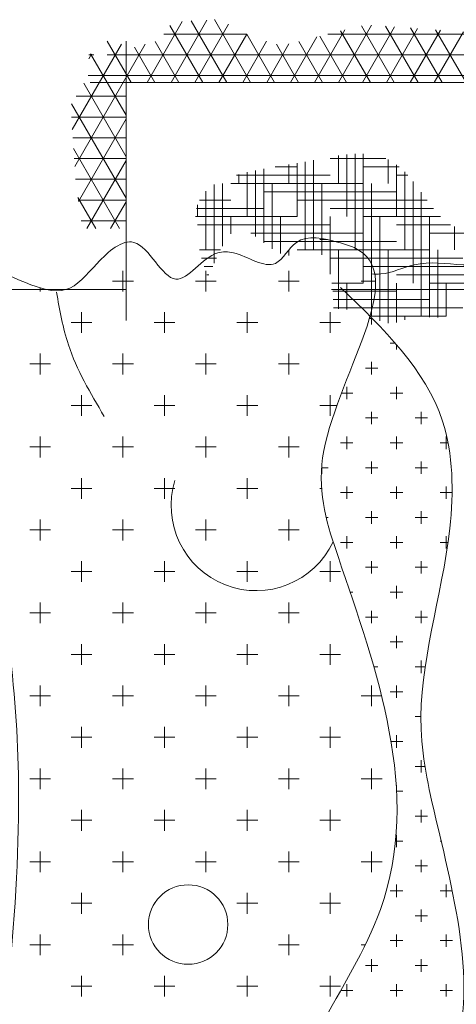
# Model space of a CAD drawing. Units: inches. Extents: x 3731 to 4318, y 1310 to 2388.
# Tile 37 of 57: x 3870 to 3897, y 2243 to 2304. Entities that reach past the tile are written whole.
import ezdxf

# ---------------------------------------------------------------- set-up
doc = ezdxf.new("R2010")
doc.units = ezdxf.units.IN
doc.layers.add('A-FURN', color=8, linetype='Continuous', lineweight=13)

# ---------------------------------------------------------------- blocks, each defined once
blk = doc.blocks.new('A$C200C7901')
for p, q in [((2, 1.6055), (2, 2.3334)), ((1.1379, 1.7195), (1.1379, 1.7508)), ((1.1222, 1.7352), (1.1535, 1.7352)), ((1.9972, 1.7352), (2.0027, 1.7352)), ((1.9972, 1.7352), (2.0027, 1.7352)), ((2, 1.6963), (2, 1.7248)), ((2, 1.6963), (2, 1.7248)), ((2.3121, 1.6596), (2.3121, 0.0201)), ((1.0129, 1.5945), (1.0129, 1.6258)), ((1.0129, 1.5945), (1.0129, 1.6258)), ((1.9533, 1.6055), (2.3741, 1.6055)), ((1.9533, 1.6055), (2.3741, 1.6055)), ((1.0754, 1.5625), (1.0754, 1.5633)), ((1.0754, 1.5625), (1.0754, 1.5633)), ((2, 0.2957), (2, 1.2957)), ((2.0224, 0.9977), (2.0224, 1.1977)), ((2.0224, 0.9977), (2.0224, 1.1977))]:
    blk.add_line(p, q)
at = {"linetype": 'ByBlock'}
for p, q in [((1.0129, 1.7195), (1.0129, 1.7508)), ((1.0129, 1.7195), (1.0129, 1.7508)), ((1.1379, 1.7195), (1.1379, 1.7508)), ((1.2629, 1.7195), (1.2629, 1.7508)), ((1.2629, 1.7195), (1.2629, 1.7508)), ((1.3879, 1.7195), (1.3879, 1.7508)), ((1.3879, 1.7195), (1.3879, 1.7508)), ((1.5129, 1.7195), (1.5129, 1.7508)), ((1.5129, 1.7195), (1.5129, 1.7508)), ((1.6379, 1.7195), (1.6379, 1.7508)), ((1.6379, 1.7195), (1.6379, 1.7508)), ((1.7629, 1.7195), (1.7629, 1.7508)), ((1.7629, 1.7195), (1.7629, 1.7508)), ((1.8879, 1.7195), (1.8879, 1.7508)), ((1.8879, 1.7195), (1.8879, 1.7508)), ((0.9972, 1.7352), (1.0285, 1.7352)), ((0.9972, 1.7352), (1.0285, 1.7352)), ((1.1222, 1.7352), (1.1535, 1.7352)), ((1.2472, 1.7352), (1.2785, 1.7352)), ((1.2472, 1.7352), (1.2785, 1.7352)), ((1.3722, 1.7352), (1.4035, 1.7352)), ((1.3722, 1.7352), (1.4035, 1.7352)), ((1.4972, 1.7352), (1.5285, 1.7352)), ((1.4972, 1.7352), (1.5285, 1.7352)), ((1.6222, 1.7352), (1.6535, 1.7352)), ((1.6222, 1.7352), (1.6535, 1.7352)), ((1.7472, 1.7352), (1.7785, 1.7352)), ((1.7472, 1.7352), (1.7785, 1.7352)), ((1.8722, 1.7352), (1.9035, 1.7352)), ((1.8722, 1.7352), (1.9035, 1.7352)), ((0.9504, 1.657), (0.9504, 1.6883)), ((0.9504, 1.657), (0.9504, 1.6883)), ((1.0754, 1.657), (1.0754, 1.6883)), ((1.0754, 1.657), (1.0754, 1.6883)), ((1.2004, 1.657), (1.2004, 1.6883)), ((1.2004, 1.657), (1.2004, 1.6883)), ((1.3254, 1.657), (1.3254, 1.6883)), ((1.3254, 1.657), (1.3254, 1.6883)), ((1.4504, 1.657), (1.4504, 1.6883)), ((1.4504, 1.657), (1.4504, 1.6883)), ((1.5754, 1.657), (1.5754, 1.6883)), ((1.5754, 1.657), (1.5754, 1.6883)), ((1.7004, 1.657), (1.7004, 1.6883)), ((1.7004, 1.657), (1.7004, 1.6883)), ((1.8254, 1.657), (1.8254, 1.6883)), ((1.8254, 1.657), (1.8254, 1.6883)), ((1.9504, 1.657), (1.9504, 1.6883)), ((1.9504, 1.657), (1.9504, 1.6883)), ((2.0919, 1.6152), (2.2125, 1.6848)), ((2.0919, 1.6152), (2.2125, 1.6848)), ((2.0919, 1.6513), (2.1386, 1.6782)), ((2.0919, 1.6513), (2.1386, 1.6782)), ((2.1327, 1.6773), (2.2571, 1.6055)), ((2.1327, 1.6773), (2.2571, 1.6055)), ((2.1349, 1.6055), (2.1349, 1.6777)), ((2.1349, 1.6055), (2.1349, 1.6777)), ((2.1377, 1.6055), (2.2798, 1.6876)), ((2.1377, 1.6055), (2.2798, 1.6876)), ((2.1662, 1.6055), (2.1662, 1.6817)), ((2.1662, 1.6055), (2.1662, 1.6817)), ((2.1854, 1.683), (2.3697, 1.5766)), ((2.1854, 1.683), (2.3697, 1.5766)), ((2.1974, 1.6055), (2.1974, 1.6838)), ((2.1974, 1.6055), (2.1974, 1.6838)), ((2.2287, 1.6055), (2.2287, 1.6859)), ((2.2287, 1.6055), (2.2287, 1.6859)), ((2.2414, 1.6868), (2.3699, 1.6126)), ((2.2414, 1.6868), (2.3699, 1.6126)), ((2.2599, 1.6055), (2.2599, 1.688)), ((2.2599, 1.6055), (2.2599, 1.688)), ((2.2912, 1.6055), (2.2912, 1.6809)), ((2.2912, 1.6055), (2.2912, 1.6809)), ((0.9347, 1.6727), (0.966, 1.6727)), ((0.9347, 1.6727), (0.966, 1.6727)), ((1.0597, 1.6727), (1.091, 1.6727)), ((1.0597, 1.6727), (1.091, 1.6727)), ((1.1847, 1.6727), (1.216, 1.6727)), ((1.1847, 1.6727), (1.216, 1.6727)), ((1.3097, 1.6727), (1.341, 1.6727)), ((1.3097, 1.6727), (1.341, 1.6727)), ((1.4347, 1.6727), (1.466, 1.6727)), ((1.4347, 1.6727), (1.466, 1.6727)), ((1.5597, 1.6727), (1.591, 1.6727)), ((1.5597, 1.6727), (1.591, 1.6727)), ((1.6847, 1.6727), (1.716, 1.6727)), ((1.6847, 1.6727), (1.716, 1.6727)), ((1.8097, 1.6727), (1.841, 1.6727)), ((1.8097, 1.6727), (1.841, 1.6727)), ((1.9347, 1.6727), (1.966, 1.6727)), ((1.9347, 1.6727), (1.966, 1.6727)), ((2.0919, 1.6649), (2.1946, 1.6055)), ((2.0919, 1.6649), (2.1946, 1.6055)), ((2.1037, 1.6055), (2.1037, 1.673)), ((2.1037, 1.6055), (2.1037, 1.673)), ((2.2002, 1.6055), (2.3109, 1.6694)), ((2.2002, 1.6055), (2.3109, 1.6694)), ((2.3224, 0.0468), (2.3224, 1.6627)), ((2.3224, 0.0468), (2.3224, 1.6627)), ((2.3476, 1.6616), (2.3547, 1.6575)), ((2.3476, 1.6616), (2.3547, 1.6575)), ((2.3537, 1.6539), (2.3537, 1.6616)), ((2.3537, 1.6539), (2.3537, 1.6616)), ((2.2627, 1.6055), (2.3551, 1.6589)), ((2.2627, 1.6055), (2.3551, 1.6589)), ((2.3121, 1.598), (2.3745, 1.634)), ((2.3121, 1.598), (2.3745, 1.634)), ((2.3537, 0.0056), (2.3537, 1.634)), ((2.3537, 0.0056), (2.3537, 1.634)), ((1.1379, 1.5945), (1.1379, 1.6258)), ((1.1379, 1.5945), (1.1379, 1.6258)), ((1.2629, 1.5945), (1.2629, 1.6258)), ((1.2629, 1.5945), (1.2629, 1.6258)), ((1.3879, 1.5945), (1.3879, 1.6258)), ((1.3879, 1.5945), (1.3879, 1.6258)), ((1.5129, 1.5945), (1.5129, 1.6258)), ((1.5129, 1.5945), (1.5129, 1.6258)), ((1.6379, 1.5945), (1.6379, 1.6258)), ((1.6379, 1.5945), (1.6379, 1.6258)), ((1.7629, 1.5945), (1.7629, 1.6258)), ((1.7629, 1.5945), (1.7629, 1.6258)), ((1.8879, 1.5945), (1.8879, 1.6258)), ((1.8879, 1.5945), (1.8879, 1.6258)), ((2.0129, 1.5945), (2.0129, 1.6258)), ((2.0129, 1.5945), (2.0129, 1.6258)), ((2.0919, 1.6288), (2.1321, 1.6055)), ((2.0919, 1.6288), (2.1321, 1.6055)), ((0.9972, 1.6102), (1.0285, 1.6102)), ((0.9972, 1.6102), (1.0285, 1.6102)), ((1.1222, 1.6102), (1.1535, 1.6102)), ((1.1222, 1.6102), (1.1535, 1.6102)), ((1.2472, 1.6102), (1.2785, 1.6102)), ((1.2472, 1.6102), (1.2785, 1.6102)), ((1.3722, 1.6102), (1.4035, 1.6102)), ((1.3722, 1.6102), (1.4035, 1.6102)), ((1.4972, 1.6102), (1.5285, 1.6102)), ((1.4972, 1.6102), (1.5285, 1.6102)), ((1.6222, 1.6102), (1.6535, 1.6102)), ((1.6222, 1.6102), (1.6535, 1.6102)), ((1.7472, 1.6102), (1.7785, 1.6102)), ((1.7472, 1.6102), (1.7785, 1.6102)), ((1.8722, 1.6102), (1.9035, 1.6102)), ((1.8722, 1.6102), (1.9035, 1.6102)), ((1.9972, 1.6102), (2.0285, 1.6102)), ((1.9972, 1.6102), (2.0285, 1.6102)), ((2.3121, 1.5619), (2.3654, 1.5926)), ((2.3121, 1.5619), (2.3654, 1.5926)), ((2.3121, 1.5738), (2.404, 1.5208)), ((2.3121, 1.5738), (2.404, 1.5208)), ((0.9504, 1.532), (0.9504, 1.5633)), ((0.9504, 1.532), (0.9504, 1.5633)), ((1.2004, 1.532), (1.2004, 1.5633)), ((1.2004, 1.532), (1.2004, 1.5633)), ((1.3254, 1.532), (1.3254, 1.5633)), ((1.3254, 1.532), (1.3254, 1.5633)), ((1.4504, 1.532), (1.4504, 1.5633)), ((1.4504, 1.532), (1.4504, 1.5633)), ((1.5754, 1.532), (1.5754, 1.5633)), ((1.5754, 1.532), (1.5754, 1.5633)), ((1.7004, 1.532), (1.7004, 1.5633)), ((1.7004, 1.532), (1.7004, 1.5633)), ((1.8254, 1.532), (1.8254, 1.5633)), ((1.8254, 1.532), (1.8254, 1.5633)), ((1.9504, 1.532), (1.9504, 1.5633)), ((1.9504, 1.532), (1.9504, 1.5633)), ((2.3121, 1.5258), (2.3739, 1.5615)), ((2.3121, 1.5258), (2.3739, 1.5615)), ((0.9347, 1.5477), (0.966, 1.5477)), ((0.9347, 1.5477), (0.966, 1.5477)), ((1.1847, 1.5477), (1.216, 1.5477)), ((1.1847, 1.5477), (1.216, 1.5477)), ((1.3097, 1.5477), (1.341, 1.5477)), ((1.3097, 1.5477), (1.341, 1.5477)), ((1.4347, 1.5477), (1.466, 1.5477)), ((1.4347, 1.5477), (1.466, 1.5477)), ((1.5597, 1.5477), (1.591, 1.5477)), ((1.5597, 1.5477), (1.591, 1.5477)), ((1.6847, 1.5477), (1.716, 1.5477)), ((1.6847, 1.5477), (1.716, 1.5477)), ((1.8097, 1.5477), (1.841, 1.5477)), ((1.8097, 1.5477), (1.841, 1.5477)), ((1.9347, 1.5477), (1.966, 1.5477)), ((1.9347, 1.5477), (1.966, 1.5477)), ((2.3849, 1.4236), (2.3849, 1.5486)), ((2.3849, 1.4236), (2.3849, 1.5486)), ((2.3121, 1.4897), (2.3979, 1.5393)), ((2.3121, 1.4897), (2.3979, 1.5393)), ((2.3121, 1.5377), (2.406, 1.4835)), ((2.3121, 1.5377), (2.406, 1.4835)), ((1.1379, 1.4695), (1.1379, 1.5008)), ((1.1379, 1.4695), (1.1379, 1.5008)), ((1.2629, 1.4695), (1.2629, 1.5008)), ((1.2629, 1.4695), (1.2629, 1.5008)), ((1.3879, 1.4695), (1.3879, 1.5008)), ((1.3879, 1.4695), (1.3879, 1.5008)), ((1.5129, 1.4695), (1.5129, 1.5008)), ((1.5129, 1.4695), (1.5129, 1.5008)), ((1.6379, 1.4695), (1.6379, 1.5008)), ((1.6379, 1.4695), (1.6379, 1.5008)), ((1.7629, 1.4695), (1.7629, 1.5008)), ((1.7629, 1.4695), (1.7629, 1.5008)), ((1.8879, 1.4695), (1.8879, 1.5008)), ((1.8879, 1.4695), (1.8879, 1.5008)), ((2.0129, 1.4695), (2.0129, 1.5008)), ((2.0129, 1.4695), (2.0129, 1.5008)), ((2.1099, 1.3477), (2.1099, 1.5009)), ((2.1099, 1.3477), (2.1099, 1.5009)), ((2.1224, 1.3977), (2.1224, 1.4992)), ((2.1224, 1.3977), (2.1224, 1.4992)), ((2.3121, 1.4537), (2.4047, 1.5071)), ((2.3121, 1.4537), (2.4047, 1.5071)), ((2.3121, 1.5016), (2.3997, 1.4511)), ((2.3121, 1.5016), (2.3997, 1.4511)), ((1.1222, 1.4852), (1.1535, 1.4852)), ((1.1222, 1.4852), (1.1535, 1.4852)), ((1.2472, 1.4852), (1.2785, 1.4852)), ((1.2472, 1.4852), (1.2785, 1.4852)), ((1.3722, 1.4852), (1.4035, 1.4852)), ((1.3722, 1.4852), (1.4035, 1.4852)), ((1.4972, 1.4852), (1.5285, 1.4852)), ((1.4972, 1.4852), (1.5285, 1.4852)), ((1.6222, 1.4852), (1.6535, 1.4852)), ((1.6222, 1.4852), (1.6535, 1.4852)), ((1.7472, 1.4852), (1.7785, 1.4852)), ((1.7472, 1.4852), (1.7785, 1.4852)), ((1.8722, 1.4852), (1.9035, 1.4852)), ((1.8722, 1.4852), (1.9035, 1.4852)), ((1.9972, 1.4852), (2.0285, 1.4852)), ((1.9972, 1.4852), (2.0285, 1.4852)), ((2.0224, 1.4805), (2.0224, 1.4839)), ((2.0224, 1.4805), (2.0224, 1.4839)), ((2.0349, 1.4748), (2.0349, 1.4879)), ((2.0349, 1.4748), (2.0349, 1.4879)), ((2.0474, 1.4691), (2.0474, 1.4915)), ((2.0474, 1.4691), (2.0474, 1.4915)), ((2.0599, 1.4631), (2.0599, 1.4948)), ((2.0599, 1.4631), (2.0599, 1.4948)), ((2.0599, 1.4852), (2.1484, 1.4852)), ((2.0599, 1.4852), (2.1484, 1.4852)), ((2.0974, 1.2977), (2.0974, 1.4977)), ((2.0974, 1.2977), (2.0974, 1.4977)), ((2.1099, 1.4977), (2.1279, 1.4977)), ((2.1099, 1.4977), (2.1279, 1.4977)), ((2.1349, 1.4477), (2.1349, 1.4949)), ((2.1349, 1.4477), (2.1349, 1.4949)), ((2.0397, 1.4727), (2.1581, 1.4727)), ((2.0397, 1.4727), (2.1581, 1.4727)), ((2.3121, 1.4176), (2.4067, 1.4721)), ((2.3121, 1.4176), (2.4067, 1.4721)), ((2.0656, 1.4602), (2.1599, 1.4602)), ((2.0656, 1.4602), (2.1599, 1.4602)), ((2.3121, 1.4655), (2.3849, 1.4235)), ((2.3121, 1.4655), (2.3849, 1.4235)), ((2.084, 1.4477), (2.1099, 1.4477)), ((2.084, 1.4477), (2.1099, 1.4477)), ((2.0849, 1.4468), (2.0849, 1.4477)), ((2.0849, 1.4468), (2.0849, 1.4477)), ((2.1599, 1.2477), (2.1599, 1.4477)), ((2.1599, 1.2477), (2.1599, 1.4477)), ((2.1724, 1.2977), (2.1724, 1.439)), ((2.1724, 1.2977), (2.1724, 1.439)), ((0.9504, 1.407), (0.9504, 1.4383)), ((0.9504, 1.407), (0.9504, 1.4383)), ((1.0754, 1.407), (1.0754, 1.4383)), ((1.0754, 1.407), (1.0754, 1.4383)), ((1.2004, 1.407), (1.2004, 1.4383)), ((1.2004, 1.407), (1.2004, 1.4383)), ((1.3254, 1.407), (1.3254, 1.4383)), ((1.3254, 1.407), (1.3254, 1.4383)), ((1.4504, 1.407), (1.4504, 1.4383)), ((1.4504, 1.407), (1.4504, 1.4383)), ((1.5754, 1.407), (1.5754, 1.4383)), ((1.5754, 1.407), (1.5754, 1.4383)), ((1.7004, 1.407), (1.7004, 1.4383)), ((1.7004, 1.407), (1.7004, 1.4383)), ((1.8254, 1.407), (1.8254, 1.4383)), ((1.8254, 1.407), (1.8254, 1.4383)), ((1.9504, 1.407), (1.9504, 1.4383)), ((1.9504, 1.407), (1.9504, 1.4383)), ((2.1599, 1.4352), (2.1735, 1.4352)), ((2.1599, 1.4352), (2.1735, 1.4352)), ((2.3121, 1.4294), (2.3741, 1.3937)), ((2.3121, 1.4294), (2.3741, 1.3937)), ((0.9347, 1.4227), (0.966, 1.4227)), ((0.9347, 1.4227), (0.966, 1.4227)), ((1.0597, 1.4227), (1.091, 1.4227)), ((1.0597, 1.4227), (1.091, 1.4227)), ((1.1847, 1.4227), (1.216, 1.4227)), ((1.1847, 1.4227), (1.216, 1.4227)), ((1.3097, 1.4227), (1.341, 1.4227)), ((1.3097, 1.4227), (1.341, 1.4227)), ((1.4347, 1.4227), (1.466, 1.4227)), ((1.4347, 1.4227), (1.466, 1.4227)), ((1.5597, 1.4227), (1.591, 1.4227)), ((1.5597, 1.4227), (1.591, 1.4227)), ((1.6847, 1.4227), (1.716, 1.4227)), ((1.6847, 1.4227), (1.716, 1.4227)), ((1.8097, 1.4227), (1.841, 1.4227)), ((1.8097, 1.4227), (1.841, 1.4227)), ((1.9347, 1.4227), (1.966, 1.4227)), ((1.9347, 1.4227), (1.966, 1.4227)), ((2.08, 1.4102), (2.1795, 1.4102)), ((2.08, 1.4102), (2.1795, 1.4102)), ((2.0849, 1.2477), (2.0849, 1.4171)), ((2.0849, 1.2477), (2.0849, 1.4171)), ((2.1099, 1.4227), (2.1767, 1.4227)), ((2.1099, 1.4227), (2.1767, 1.4227)), ((2.3121, 1.3815), (2.3848, 1.4235)), ((2.3121, 1.3815), (2.3848, 1.4235)), ((2.0703, 1.3977), (2.1819, 1.3977)), ((2.0703, 1.3977), (2.1819, 1.3977)), ((2.0724, 1.1977), (2.0724, 1.3977)), ((2.0724, 1.1977), (2.0724, 1.3977)), ((2.1474, 1.1977), (2.1474, 1.3977)), ((2.1474, 1.1977), (2.1474, 1.3977)), ((2.0612, 1.3852), (2.1599, 1.3852)), ((2.0612, 1.3852), (2.1599, 1.3852)), ((2.1849, 1.3477), (2.1849, 1.3808)), ((2.1849, 1.3477), (2.1849, 1.3808)), ((2.3121, 1.3934), (2.3703, 1.3598)), ((2.3121, 1.3934), (2.3703, 1.3598)), ((1.0129, 1.3445), (1.0129, 1.3758)), ((1.0129, 1.3445), (1.0129, 1.3758)), ((1.1379, 1.3445), (1.1379, 1.3758)), ((1.1379, 1.3445), (1.1379, 1.3758)), ((1.2629, 1.3445), (1.2629, 1.3758)), ((1.2629, 1.3445), (1.2629, 1.3758)), ((1.3879, 1.3445), (1.3879, 1.3758)), ((1.3879, 1.3445), (1.3879, 1.3758)), ((1.5129, 1.3445), (1.5129, 1.3758)), ((1.5129, 1.3445), (1.5129, 1.3758)), ((1.6379, 1.3445), (1.6379, 1.3758)), ((1.6379, 1.3445), (1.6379, 1.3758)), ((1.7629, 1.3445), (1.7629, 1.3758)), ((1.7629, 1.3445), (1.7629, 1.3758)), ((1.8879, 1.3445), (1.8879, 1.3758)), ((1.8879, 1.3445), (1.8879, 1.3758)), ((2.0129, 1.3445), (2.0129, 1.3758)), ((2.0129, 1.3445), (2.0129, 1.3758)), ((2.0545, 1.3727), (2.1099, 1.3727)), ((2.0545, 1.3727), (2.1099, 1.3727)), ((2.3121, 1.3454), (2.37, 1.3788)), ((2.3121, 1.3454), (2.37, 1.3788)), ((0.9972, 1.3602), (1.0285, 1.3602)), ((0.9972, 1.3602), (1.0285, 1.3602)), ((1.1222, 1.3602), (1.1535, 1.3602)), ((1.1222, 1.3602), (1.1535, 1.3602)), ((1.2472, 1.3602), (1.2785, 1.3602)), ((1.2472, 1.3602), (1.2785, 1.3602)), ((1.3722, 1.3602), (1.4035, 1.3602)), ((1.3722, 1.3602), (1.4035, 1.3602)), ((1.4972, 1.3602), (1.5285, 1.3602)), ((1.4972, 1.3602), (1.5285, 1.3602)), ((1.6222, 1.3602), (1.6535, 1.3602)), ((1.6222, 1.3602), (1.6535, 1.3602)), ((1.7472, 1.3602), (1.7785, 1.3602)), ((1.7472, 1.3602), (1.7785, 1.3602)), ((1.8722, 1.3602), (1.9035, 1.3602)), ((1.8722, 1.3602), (1.9035, 1.3602)), ((1.9972, 1.3602), (2.0285, 1.3602)), ((1.9972, 1.3602), (2.0285, 1.3602)), ((2.0515, 1.3602), (2.0599, 1.3602)), ((2.0515, 1.3602), (2.0599, 1.3602)), ((2.1599, 1.3602), (2.1883, 1.3602)), ((2.1599, 1.3602), (2.1883, 1.3602)), ((2.3121, 1.3573), (2.3808, 1.3176)), ((2.3121, 1.3573), (2.3808, 1.3176)), ((2.0599, 1.1477), (2.0599, 1.3477)), ((2.0599, 1.1477), (2.0599, 1.3477)), ((2.0599, 1.3352), (2.1926, 1.3352)), ((2.0599, 1.3352), (2.1926, 1.3352)), ((2.1099, 1.3477), (2.1904, 1.3477)), ((2.1099, 1.3477), (2.1904, 1.3477)), ((2.1349, 1.1515), (2.1349, 1.3477)), ((2.1349, 1.1515), (2.1349, 1.3477)), ((2.3121, 1.3093), (2.374, 1.345)), ((2.3121, 1.3093), (2.374, 1.345)), ((2.0594, 1.3227), (2.195, 1.3227)), ((2.0594, 1.3227), (2.195, 1.3227)), ((2.3121, 1.3212), (2.3914, 1.2754)), ((2.3121, 1.3212), (2.3914, 1.2754)), ((0.9504, 1.282), (0.9504, 1.3133)), ((0.9504, 1.282), (0.9504, 1.3133)), ((1.0754, 1.282), (1.0754, 1.3133)), ((1.0754, 1.282), (1.0754, 1.3133)), ((1.2004, 1.282), (1.2004, 1.3133)), ((1.2004, 1.282), (1.2004, 1.3133)), ((1.3254, 1.282), (1.3254, 1.3133)), ((1.3254, 1.282), (1.3254, 1.3133)), ((1.4504, 1.282), (1.4504, 1.3133)), ((1.4504, 1.282), (1.4504, 1.3133)), ((1.5754, 1.282), (1.5754, 1.3133)), ((1.5754, 1.282), (1.5754, 1.3133)), ((1.7004, 1.3106), (1.7004, 1.3133)), ((1.7004, 1.3106), (1.7004, 1.3133)), ((1.7222, 1.3102), (1.7369, 1.3102)), ((1.7222, 1.3102), (1.7369, 1.3102)), ((1.7316, 1.3008), (1.7316, 1.3106)), ((1.7316, 1.3008), (1.7316, 1.3106)), ((1.8254, 1.2876), (1.8254, 1.3133)), ((1.8254, 1.2876), (1.8254, 1.3133)), ((1.9504, 1.282), (1.9504, 1.3133)), ((1.9504, 1.282), (1.9504, 1.3133)), ((2.0524, 1.3102), (2.1599, 1.3102)), ((2.0524, 1.3102), (2.1599, 1.3102)), ((2.0754, 1.3017), (2.0754, 1.3133)), ((2.0754, 1.3017), (2.0754, 1.3133)), ((2.3121, 1.2732), (2.3819, 1.3135)), ((2.3121, 1.2732), (2.3819, 1.3135)), ((0.9347, 1.2977), (0.966, 1.2977)), ((0.9347, 1.2977), (0.966, 1.2977)), ((1.0597, 1.2977), (1.091, 1.2977)), ((1.0597, 1.2977), (1.091, 1.2977)), ((1.1847, 1.2977), (1.216, 1.2977)), ((1.1847, 1.2977), (1.216, 1.2977)), ((1.3097, 1.2977), (1.341, 1.2977)), ((1.3097, 1.2977), (1.341, 1.2977)), ((1.4347, 1.2977), (1.466, 1.2977)), ((1.4347, 1.2977), (1.466, 1.2977)), ((1.5597, 1.2977), (1.591, 1.2977)), ((1.5597, 1.2977), (1.591, 1.2977)), ((1.6566, 1.3008), (1.6566, 1.3036)), ((1.6566, 1.3008), (1.6566, 1.3036)), ((1.8097, 1.2977), (1.841, 1.2977)), ((1.8097, 1.2977), (1.841, 1.2977)), ((1.9347, 1.2977), (1.966, 1.2977)), ((1.9347, 1.2977), (1.966, 1.2977)), ((1.9724, 1.0977), (1.9724, 1.2927)), ((1.9724, 1.0977), (1.9724, 1.2927)), ((1.9849, 1.1477), (1.9849, 1.293)), ((1.9849, 1.1477), (1.9849, 1.293)), ((1.9974, 1.1977), (1.9974, 1.2939)), ((1.9974, 1.1977), (1.9974, 1.2939)), ((2.0099, 1.2477), (2.0099, 1.2953)), ((2.0099, 1.2477), (2.0099, 1.2953)), ((2.023, 1.2977), (2.1099, 1.2977)), ((2.023, 1.2977), (2.1099, 1.2977)), ((2.0474, 1.0977), (2.0474, 1.2977)), ((2.0474, 1.0977), (2.0474, 1.2977)), ((2.0597, 1.2977), (2.0744, 1.2977)), ((2.0597, 1.2977), (2.0744, 1.2977)), ((2.1224, 1.1421), (2.1224, 1.2977)), ((2.1224, 1.1421), (2.1224, 1.2977)), ((2.1974, 1.2135), (2.1974, 1.2977)), ((2.1974, 1.2135), (2.1974, 1.2977)), ((2.3849, 1.0607), (2.3849, 1.3013)), ((2.3849, 1.0607), (2.3849, 1.3013)), ((0.9441, 1.2633), (0.9441, 1.2816)), ((0.9441, 1.2633), (0.9441, 1.2816)), ((1.6191, 1.2633), (1.6191, 1.282)), ((1.6191, 1.2633), (1.6191, 1.282)), ((1.6941, 1.2633), (1.6941, 1.282)), ((1.6941, 1.2633), (1.6941, 1.282)), ((1.7691, 1.2633), (1.7691, 1.282)), ((1.7691, 1.2633), (1.7691, 1.282)), ((1.8441, 1.2633), (1.8441, 1.2806)), ((1.8441, 1.2633), (1.8441, 1.2806)), ((1.9711, 1.2852), (2.0599, 1.2852)), ((1.9711, 1.2852), (2.0599, 1.2852)), ((2.1599, 1.2852), (2.2018, 1.2852)), ((2.1599, 1.2852), (2.2018, 1.2852)), ((2.3121, 1.2851), (2.3985, 1.2352)), ((2.3121, 1.2851), (2.3985, 1.2352)), ((2.3121, 1.2371), (2.3898, 1.282)), ((2.3121, 1.2371), (2.3898, 1.282)), ((0.9347, 1.2727), (0.9535, 1.2727)), ((0.9347, 1.2727), (0.9535, 1.2727)), ((1.5441, 1.2633), (1.5441, 1.2675)), ((1.5441, 1.2633), (1.5441, 1.2675)), ((1.6097, 1.2727), (1.6285, 1.2727)), ((1.6097, 1.2727), (1.6285, 1.2727)), ((1.6847, 1.2727), (1.7035, 1.2727)), ((1.6847, 1.2727), (1.7035, 1.2727)), ((1.7597, 1.2727), (1.7785, 1.2727)), ((1.7597, 1.2727), (1.7785, 1.2727)), ((1.8347, 1.2727), (1.8535, 1.2727)), ((1.8347, 1.2727), (1.8535, 1.2727)), ((1.97, 1.2727), (2.0099, 1.2727)), ((1.97, 1.2727), (2.0099, 1.2727)), ((2.1099, 1.2727), (2.2034, 1.2727)), ((2.1099, 1.2727), (2.2034, 1.2727)), ((1.0129, 1.2448), (1.0129, 1.2508)), ((1.0129, 1.2448), (1.0129, 1.2508)), ((1.1379, 1.2195), (1.1379, 1.2508)), ((1.1379, 1.2195), (1.1379, 1.2508)), ((1.2629, 1.2195), (1.2629, 1.2508)), ((1.2629, 1.2195), (1.2629, 1.2508)), ((1.3879, 1.2202), (1.3879, 1.2508)), ((1.3879, 1.2202), (1.3879, 1.2508)), ((2.0099, 1.2477), (2.2045, 1.2477)), ((2.0099, 1.2477), (2.2045, 1.2477)), ((2.0129, 1.2293), (2.0129, 1.2508)), ((2.0129, 1.2293), (2.0129, 1.2508)), ((2.0349, 1.0477), (2.0349, 1.2477)), ((2.0349, 1.0477), (2.0349, 1.2477)), ((2.0599, 1.2602), (2.2044, 1.2602)), ((2.0599, 1.2602), (2.2044, 1.2602)), ((2.1099, 1.1315), (2.1099, 1.2477)), ((2.1099, 1.1315), (2.1099, 1.2477)), ((2.1849, 1.1935), (2.1849, 1.2477)), ((2.1849, 1.1935), (2.1849, 1.2477)), ((2.3121, 1.2011), (2.3976, 1.2504)), ((2.3121, 1.2011), (2.3976, 1.2504)), ((2.3121, 1.249), (2.396, 1.2006)), ((2.3121, 1.249), (2.396, 1.2006)), ((0.9722, 1.2352), (0.991, 1.2352)), ((0.9722, 1.2352), (0.991, 1.2352)), ((0.9816, 1.2258), (0.9816, 1.2445)), ((0.9816, 1.2258), (0.9816, 1.2445)), ((1.1222, 1.2352), (1.1535, 1.2352)), ((1.1222, 1.2352), (1.1535, 1.2352)), ((1.2472, 1.2352), (1.2785, 1.2352)), ((1.2472, 1.2352), (1.2785, 1.2352)), ((1.3722, 1.2352), (1.4035, 1.2352)), ((1.3722, 1.2352), (1.4035, 1.2352)), ((1.4316, 1.2258), (1.4316, 1.2318)), ((1.4316, 1.2258), (1.4316, 1.2318)), ((1.4972, 1.2352), (1.516, 1.2352)), ((1.4972, 1.2352), (1.516, 1.2352)), ((1.5066, 1.2258), (1.5066, 1.2445)), ((1.5066, 1.2258), (1.5066, 1.2445)), ((1.5722, 1.2352), (1.591, 1.2352)), ((1.5722, 1.2352), (1.591, 1.2352)), ((1.5816, 1.2258), (1.5816, 1.2445)), ((1.5816, 1.2258), (1.5816, 1.2445)), ((1.6472, 1.2352), (1.666, 1.2352)), ((1.6472, 1.2352), (1.666, 1.2352)), ((1.6566, 1.2258), (1.6566, 1.2445)), ((1.6566, 1.2258), (1.6566, 1.2445)), ((1.7222, 1.2352), (1.741, 1.2352)), ((1.7222, 1.2352), (1.741, 1.2352)), ((1.7316, 1.2258), (1.7316, 1.2445)), ((1.7316, 1.2258), (1.7316, 1.2445)), ((1.7972, 1.2352), (1.816, 1.2352)), ((1.7972, 1.2352), (1.816, 1.2352)), ((1.8066, 1.2258), (1.8066, 1.2445)), ((1.8066, 1.2258), (1.8066, 1.2445)), ((1.8722, 1.2352), (1.891, 1.2352)), ((1.8722, 1.2352), (1.891, 1.2352)), ((1.8816, 1.2258), (1.8816, 1.2445)), ((1.8816, 1.2258), (1.8816, 1.2445)), ((1.9472, 1.2352), (1.9574, 1.2352)), ((1.9472, 1.2352), (1.9574, 1.2352)), ((1.9566, 1.2344), (1.9566, 1.2385)), ((1.9566, 1.2344), (1.9566, 1.2385)), ((1.9599, 1.1228), (1.9599, 1.2373)), ((1.9599, 1.1228), (1.9599, 1.2373)), ((1.9599, 1.2352), (2.1599, 1.2352)), ((1.9599, 1.2352), (2.1599, 1.2352)), ((2, 1.2352), (2.0285, 1.2352)), ((2, 1.2352), (2.0285, 1.2352)), ((1.953, 1.2227), (2.1099, 1.2227)), ((1.953, 1.2227), (2.1099, 1.2227)), ((0.9441, 1.1883), (0.9441, 1.207)), ((0.9441, 1.1883), (0.9441, 1.207)), ((1.0191, 1.1883), (1.0191, 1.207)), ((1.0191, 1.1883), (1.0191, 1.207)), ((1.0941, 1.1883), (1.0941, 1.207)), ((1.0941, 1.1883), (1.0941, 1.207)), ((1.3191, 1.1883), (1.3191, 1.2059)), ((1.3191, 1.1883), (1.3191, 1.2059)), ((1.3941, 1.1883), (1.3941, 1.207)), ((1.3941, 1.1883), (1.3941, 1.207)), ((1.4691, 1.1883), (1.4691, 1.207)), ((1.4691, 1.1883), (1.4691, 1.207)), ((1.5441, 1.1883), (1.5441, 1.207)), ((1.5441, 1.1883), (1.5441, 1.207)), ((1.6191, 1.1883), (1.6191, 1.207)), ((1.6191, 1.1883), (1.6191, 1.207)), ((1.6941, 1.1883), (1.6941, 1.207)), ((1.6941, 1.1883), (1.6941, 1.207)), ((1.7691, 1.1883), (1.7691, 1.207)), ((1.7691, 1.1883), (1.7691, 1.207)), ((1.8441, 1.1883), (1.8441, 1.207)), ((1.8441, 1.1883), (1.8441, 1.207)), ((1.9191, 1.1995), (1.9191, 1.207)), ((1.9191, 1.1995), (1.9191, 1.207)), ((1.9495, 1.2102), (2.0599, 1.2102)), ((1.9495, 1.2102), (2.0599, 1.2102)), ((2.1599, 1.2102), (2.1959, 1.2102)), ((2.1599, 1.2102), (2.1959, 1.2102)), ((2.3121, 1.165), (2.397, 1.214)), ((2.3121, 1.165), (2.397, 1.214)), ((2.3121, 1.2129), (2.3935, 1.166)), ((2.3121, 1.2129), (2.3935, 1.166)), ((0.9347, 1.1977), (0.9535, 1.1977)), ((0.9347, 1.1977), (0.9535, 1.1977)), ((1.0097, 1.1977), (1.0285, 1.1977)), ((1.0097, 1.1977), (1.0285, 1.1977)), ((1.0847, 1.1977), (1.1035, 1.1977)), ((1.0847, 1.1977), (1.1035, 1.1977)), ((1.1597, 1.1977), (1.1785, 1.1977)), ((1.1597, 1.1977), (1.1785, 1.1977)), ((1.1691, 1.1883), (1.1691, 1.1991)), ((1.1691, 1.1883), (1.1691, 1.1991)), ((1.2441, 1.1883), (1.2441, 1.1976)), ((1.2441, 1.1883), (1.2441, 1.1976)), ((1.2452, 1.1977), (1.2535, 1.1977)), ((1.2452, 1.1977), (1.2535, 1.1977)), ((1.3097, 1.1977), (1.3285, 1.1977)), ((1.3097, 1.1977), (1.3285, 1.1977)), ((1.3847, 1.1977), (1.4035, 1.1977)), ((1.3847, 1.1977), (1.4035, 1.1977)), ((1.4597, 1.1977), (1.4785, 1.1977)), ((1.4597, 1.1977), (1.4785, 1.1977)), ((1.5347, 1.1977), (1.5535, 1.1977)), ((1.5347, 1.1977), (1.5535, 1.1977)), ((1.6097, 1.1977), (1.6285, 1.1977)), ((1.6097, 1.1977), (1.6285, 1.1977)), ((1.6847, 1.1977), (1.7035, 1.1977)), ((1.6847, 1.1977), (1.7035, 1.1977)), ((1.7597, 1.1977), (1.7785, 1.1977)), ((1.7597, 1.1977), (1.7785, 1.1977)), ((1.8347, 1.1977), (1.8535, 1.1977)), ((1.8347, 1.1977), (1.8535, 1.1977)), ((1.9097, 1.1977), (1.917, 1.1977)), ((1.9097, 1.1977), (1.917, 1.1977)), ((1.9506, 1.1977), (2.0099, 1.1977)), ((1.9506, 1.1977), (2.0099, 1.1977)), ((2.0974, 1.1161), (2.0974, 1.1977)), ((2.0974, 1.1161), (2.0974, 1.1977)), ((2.1099, 1.1977), (2.1882, 1.1977)), ((2.1099, 1.1977), (2.1882, 1.1977)), ((2.1724, 1.1807), (2.1724, 1.1977)), ((2.1724, 1.1807), (2.1724, 1.1977)), ((1.9545, 1.1852), (1.9599, 1.1852)), ((1.9545, 1.1852), (1.9599, 1.1852)), ((2.0099, 1.1727), (2.1631, 1.1727)), ((2.0099, 1.1727), (2.1631, 1.1727)), ((2.0599, 1.1852), (2.1772, 1.1852)), ((2.0599, 1.1852), (2.1772, 1.1852)), ((2.3121, 1.1768), (2.3909, 1.1314)), ((2.3121, 1.1768), (2.3909, 1.1314)), ((2.3121, 1.1289), (2.3942, 1.1763)), ((2.3121, 1.1289), (2.3942, 1.1763)), ((0.9722, 1.1602), (0.991, 1.1602)), ((0.9722, 1.1602), (0.991, 1.1602)), ((0.9816, 1.1508), (0.9816, 1.1695)), ((0.9816, 1.1508), (0.9816, 1.1695)), ((1.0472, 1.1602), (1.066, 1.1602)), ((1.0472, 1.1602), (1.066, 1.1602)), ((1.0566, 1.1508), (1.0566, 1.1695)), ((1.0566, 1.1508), (1.0566, 1.1695)), ((1.1222, 1.1602), (1.141, 1.1602)), ((1.1222, 1.1602), (1.141, 1.1602)), ((1.1316, 1.1508), (1.1316, 1.1695)), ((1.1316, 1.1508), (1.1316, 1.1695)), ((1.1972, 1.1602), (1.216, 1.1602)), ((1.1972, 1.1602), (1.216, 1.1602)), ((1.2066, 1.1508), (1.2066, 1.1695)), ((1.2066, 1.1508), (1.2066, 1.1695)), ((1.2722, 1.1602), (1.291, 1.1602)), ((1.2722, 1.1602), (1.291, 1.1602)), ((1.2816, 1.1547), (1.2816, 1.1695)), ((1.2816, 1.1547), (1.2816, 1.1695)), ((1.3566, 1.1608), (1.3566, 1.1695)), ((1.3566, 1.1608), (1.3566, 1.1695)), ((1.4222, 1.1602), (1.441, 1.1602)), ((1.4222, 1.1602), (1.441, 1.1602)), ((1.4316, 1.1544), (1.4316, 1.1695)), ((1.4316, 1.1544), (1.4316, 1.1695)), ((1.4972, 1.1602), (1.516, 1.1602)), ((1.4972, 1.1602), (1.516, 1.1602)), ((1.5066, 1.1508), (1.5066, 1.1695)), ((1.5066, 1.1508), (1.5066, 1.1695)), ((1.5722, 1.1602), (1.591, 1.1602)), ((1.5722, 1.1602), (1.591, 1.1602)), ((1.5816, 1.1508), (1.5816, 1.1695)), ((1.5816, 1.1508), (1.5816, 1.1695)), ((1.6472, 1.1602), (1.666, 1.1602)), ((1.6472, 1.1602), (1.666, 1.1602)), ((1.6566, 1.1508), (1.6566, 1.1695)), ((1.6566, 1.1508), (1.6566, 1.1695)), ((1.7222, 1.1602), (1.741, 1.1602)), ((1.7222, 1.1602), (1.741, 1.1602)), ((1.7316, 1.1508), (1.7316, 1.1695)), ((1.7316, 1.1508), (1.7316, 1.1695)), ((1.7972, 1.1602), (1.816, 1.1602)), ((1.7972, 1.1602), (1.816, 1.1602)), ((1.8066, 1.1508), (1.8066, 1.1695)), ((1.8066, 1.1508), (1.8066, 1.1695)), ((1.9599, 1.1602), (2.1468, 1.1602)), ((1.9599, 1.1602), (2.1468, 1.1602)), ((1.9585, 1.1477), (2.1099, 1.1477)), ((1.9585, 1.1477), (2.1099, 1.1477)), ((2.0099, 0.9477), (2.0099, 1.1477)), ((2.0099, 0.9477), (2.0099, 1.1477)), ((2.0849, 0.9477), (2.0849, 1.1477)), ((2.0849, 0.9477), (2.0849, 1.1477)), ((0.9441, 1.1133), (0.9441, 1.132)), ((0.9441, 1.1133), (0.9441, 1.132)), ((1.0191, 1.1133), (1.0191, 1.132)), ((1.0191, 1.1133), (1.0191, 1.132)), ((1.0941, 1.1136), (1.0941, 1.132)), ((1.0941, 1.1136), (1.0941, 1.132)), ((1.1691, 1.1303), (1.1691, 1.132)), ((1.1691, 1.1303), (1.1691, 1.132)), ((1.6191, 1.1201), (1.6191, 1.132)), ((1.6191, 1.1201), (1.6191, 1.132)), ((1.6941, 1.1139), (1.6941, 1.132)), ((1.6941, 1.1139), (1.6941, 1.132)), ((1.7691, 1.1198), (1.7691, 1.132)), ((1.7691, 1.1198), (1.7691, 1.132)), ((1.9581, 1.1352), (2.0599, 1.1352)), ((1.9581, 1.1352), (2.0599, 1.1352)), ((2.3121, 1.1408), (2.3884, 1.0967)), ((2.3121, 1.1408), (2.3884, 1.0967)), ((2.3121, 1.0928), (2.3915, 1.1386)), ((2.3121, 1.0928), (2.3915, 1.1386)), ((0.9347, 1.1227), (0.9535, 1.1227)), ((0.9347, 1.1227), (0.9535, 1.1227)), ((1.0097, 1.1227), (1.0285, 1.1227)), ((1.0097, 1.1227), (1.0285, 1.1227)), ((1.0847, 1.1227), (1.1035, 1.1227)), ((1.0847, 1.1227), (1.1035, 1.1227)), ((1.6097, 1.1227), (1.6285, 1.1227)), ((1.6097, 1.1227), (1.6285, 1.1227)), ((1.6847, 1.1227), (1.7035, 1.1227)), ((1.6847, 1.1227), (1.7035, 1.1227)), ((1.7597, 1.1227), (1.7785, 1.1227)), ((1.7597, 1.1227), (1.7785, 1.1227)), ((1.9599, 1.1227), (2.0099, 1.1227)), ((1.9599, 1.1227), (2.0099, 1.1227)), ((2.0599, 1.1102), (2.0951, 1.1102)), ((2.0599, 1.1102), (2.0951, 1.1102))]:
    blk.add_line(p, q, dxfattribs=at)
blk.add_circle((1.0433, 1.5119), 0.0599)
blk.add_arc((1.6746, 1.4093), 0.1282, 72.7909, 244.8695, dxfattribs=at)
blk.add_arc((1.6746, 1.4093), 0.1282, 72.7909, 244.8695, dxfattribs=at)
for points, knots in [([(0.4485, 1.7835), (0.4321, 1.7496), (0.4062, 1.6964), (0.49, 1.6713), (0.4719, 1.5969), (0.4123, 1.592), (0.4233, 1.5337), (0.4954, 1.5086), (0.4012, 1.4738), (0.3253, 1.4306), (0.4113, 1.3764), (0.3688, 1.3065), (0.5579, 1.2663), (0.741, 1.4533), (1.1127, 1.1109), (1.4811, 1.2478), (1.7885, 1.3492), (2.0357, 1.1637), (2.0748, 1.2974), (2.0876, 1.349), (2.0192, 1.3805), (2.0564, 1.4298), (2.0588, 1.4846), (1.9759, 1.5349), (2.1004, 1.5845), (2.0397, 1.6519), (1.971, 1.7053), (2.1104, 1.8981), (1.5946, 1.7967), (1.2448, 1.7472), (0.8129, 1.7935), (0.4953, 1.8548), (0.4582, 1.7983), (0.4485, 1.7835)], [0, 0, 0, 0, 88.420092, 139.08588, 204.302936, 239.695496, 287.801042, 327.365471, 412.960499, 463.626286, 552.059846, 584.668336, 662.614915, 940.993281, 1309.926334, 1844.022653, 1996.276242, 2316.43048, 2341.441004, 2404.707416, 2449.463774, 2514.680778, 2538.40571, 2613.031547, 2697.13096, 2760.903931, 2822.692699, 2945.47, 3215.060018, 3725.584917, 4361.974444, 4504.671998, 4555.32777, 4555.32777, 4555.32777, 4555.32777]), ([(0.4856, 1.3429), (0.5504, 1.3182), (0.6715, 1.2721), (0.8374, 1.0498), (1.1164, 1.1183), (1.3878, 1.1816), (1.5888, 1.1102), (1.8403, 1.1127), (1.9415, 1.2178), (2.0032, 1.2819)], [0, 0, 0, 0, 205.411753, 383.654933, 772.067458, 921.644661, 1226.793228, 1388.983508, 1642.292305, 1642.292305, 1642.292305, 1642.292305])]:
    blk.add_open_spline(points, degree=3, knots=knots)
for points, knots in [([(1.996, 1.7104), (1.9692, 1.7057), (1.9025, 1.6938), (1.844, 1.6592), (1.809, 1.6385)], [0, 0, 0, 0, 81.132613, 201.738644, 201.738644, 201.738644, 201.738644]), ([(1.996, 1.7104), (1.9692, 1.7057), (1.9025, 1.6938), (1.844, 1.6592), (1.809, 1.6385)], [0, 0, 0, 0, 81.132613, 201.738644, 201.738644, 201.738644, 201.738644]), ([(0.473, 1.2954), (0.4739, 1.2781), (0.4755, 1.2477), (0.5032, 1.2084), (0.4801, 1.1701), (0.4928, 1.1255), (0.4674, 1.0912), (0.4579, 1.0351), (0.501, 0.9724), (0.4311, 0.8832), (0.4902, 0.8637), (0.4843, 0.8288), (0.4774, 0.7906), (0.4625, 0.7457), (0.459, 0.6999), (0.4816, 0.6664), (0.4748, 0.625), (0.4791, 0.5889), (0.4533, 0.5528), (0.4738, 0.5004), (0.4658, 0.4502), (0.4696, 0.3946), (0.4189, 0.3935), (0.4493, 0.3684), (0.4694, 0.3857), (0.4922, 0.3576), (0.5297, 0.3262), (0.5917, 0.3353), (0.6454, 0.3754), (0.7083, 0.3741), (0.7643, 0.3328), (0.826, 0.346), (0.925, 0.3388), (1.0353, 0.3593), (1.1561, 0.3744), (1.2477, 0.3154), (1.3302, 0.3474), (1.4086, 0.3512), (1.5217, 0.3878), (1.6362, 0.3176), (1.7682, 0.3285), (1.8402, 0.3019), (1.9071, 0.3529), (1.9647, 0.3412), (2.0795, 0.2948), (2.0472, 0.3498), (2.0343, 0.3772), (2.0435, 0.43), (2.0109, 0.5782), (2.0746, 0.4643), (2.0805, 0.584), (2.0084, 0.5979), (2.0343, 0.6846), (2.0344, 0.746), (2.0293, 0.8096), (2.0489, 0.8545), (2.0652, 0.9218), (1.9842, 0.9297), (2.0007, 1.0162), (2.0367, 1.0585), (2.0367, 1.1102), (2.0457, 1.1647), (2.0226, 1.2084), (2.0234, 1.2306), (2.0236, 1.2352)], [0, 0, 0, 0, 51.660678, 90.967412, 128.902454, 170.303599, 219.852997, 247.834962, 336.321557, 429.35469, 458.821847, 477.222321, 524.135809, 581.038434, 617.839381, 657.146115, 693.947125, 740.178081, 760.753248, 820.731705, 885.133458, 928.777044, 953.563729, 976.574207, 995.553042, 1018.563482, 1064.584401, 1147.951297, 1174.787598, 1266.851571, 1308.018447, 1377.066427, 1441.511314, 1608.245014, 1714.11869, 1792.771707, 1913.247991, 1954.931389, 2029.864445, 2259.189419, 2305.221512, 2429.507982, 2456.344283, 2543.92595, 2627.925037, 2662.96218, 2687.736879, 2719.937755, 2839.540991, 2875.47895, 2953.681041, 2993.270313, 3066.872333, 3154.395764, 3200.397042, 3248.426375, 3312.828127, 3347.881398, 3444.484026, 3481.577522, 3518.665244, 3592.267265, 3644.719162, 3658.519501, 3658.519501, 3658.519501, 3658.519501])]:
    blk.add_open_spline(points, degree=3, knots=knots, dxfattribs=at)

msp = doc.modelspace()

# ---------------------------------------------------------------- block references
at = {"layer": 'A-FURN', "xscale": 41.1071563136412, "yscale": 41.1071563136412, "zscale": 41.1071563136412, "rotation": 90}
msp.add_blockref('A$C200C7901', (3942.346, 2204.601), dxfattribs=at)

doc.saveas('drawing.dxf')
